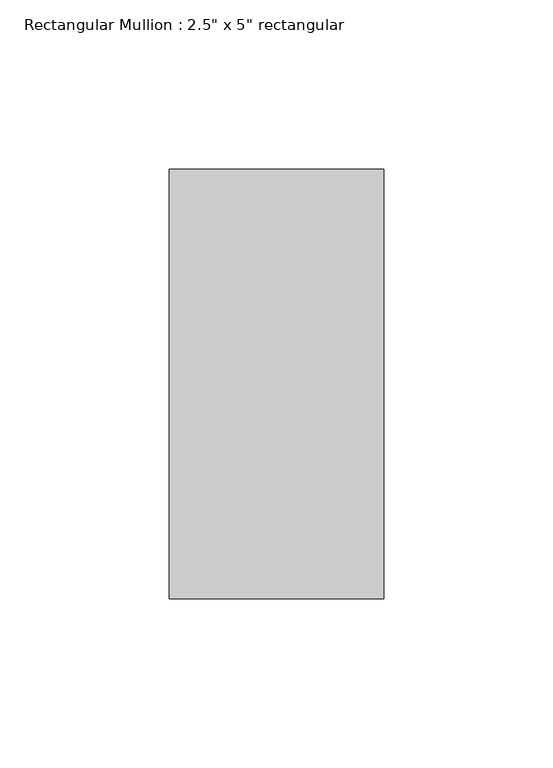
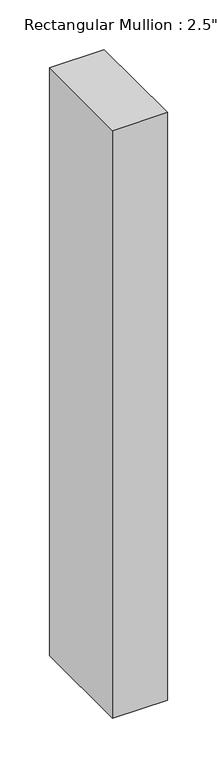
"""IFC4 building model written with IfcOpenShell, lengths in millimetres: member geometry."""

from ifc_helpers import new_model, si_unit, frame, origin, place, context, project, spatial, polyline, outline, extrude, source, transform, mapped, element, save


def member_1cc7c027(model_context):
    return source(origin(), model_context, "Body", "SweptSolid", [
        extrude(outline(polyline([(31.75, 63.5), (31.75, -63.5), (-31.75, -63.5), (-31.75, 63.5), (31.75, 63.5)])), frame((0.0, 0.0, -721.1902035), z_axis=(0.0, 0.0, 1.0), x_axis=(1.0, 0.0, 0.0)), (0.0, 0.0, 1.0), 721.1902035),
    ])


if __name__ == "__main__":
    model = new_model("IFC4")
    model_context = context("Model", 3, world=origin())
    ifc_project = project(units=[si_unit("LENGTHUNIT", "METRE", prefix="MILLI")], contexts=[model_context])
    site = spatial("IfcSite", under=ifc_project)
    building = spatial("IfcBuilding", under=site)
    placement = place(None, origin())
    member_shape = member_1cc7c027(model_context)
    element("IfcMember", 1, ObjectType="Rectangular Mullion : 2.5\" x 5\" rectangular", at=placement, inside=building, context=model_context, shape_type="MappedRepresentation", body=[
        mapped(member_shape, transform((0.0, 0.0, 0.0), x_axis=(1.0, 0.0, 0.0), y_axis=(0.0, 1.0, 0.0), z_axis=(0.0, 0.0, 1.0))),
    ])
    save(model, "model.ifc")

# Revit data of these elements
# Type "Rectangular Mullion : 2.5\" x 5\" rectangular"
#   built-in parameter 1007304 = 0.416667 (stored number, unit not read)
#   built-in parameter 1007301 = 0.104167 (stored number, unit not read)
#   built-in parameter 1007300 = 0.104167 (stored number, unit not read)
# Element 1 (IfcMember, "Rectangular Mullion : 2.5\" x 5\" rectangular")
#   Materials on its faces: "Aluminum"
# Materials
#   "Aluminum": class "Metal", colour RGB 247 247 247, transparency 0, Description = "Aluminum 6061", Cost = 0
